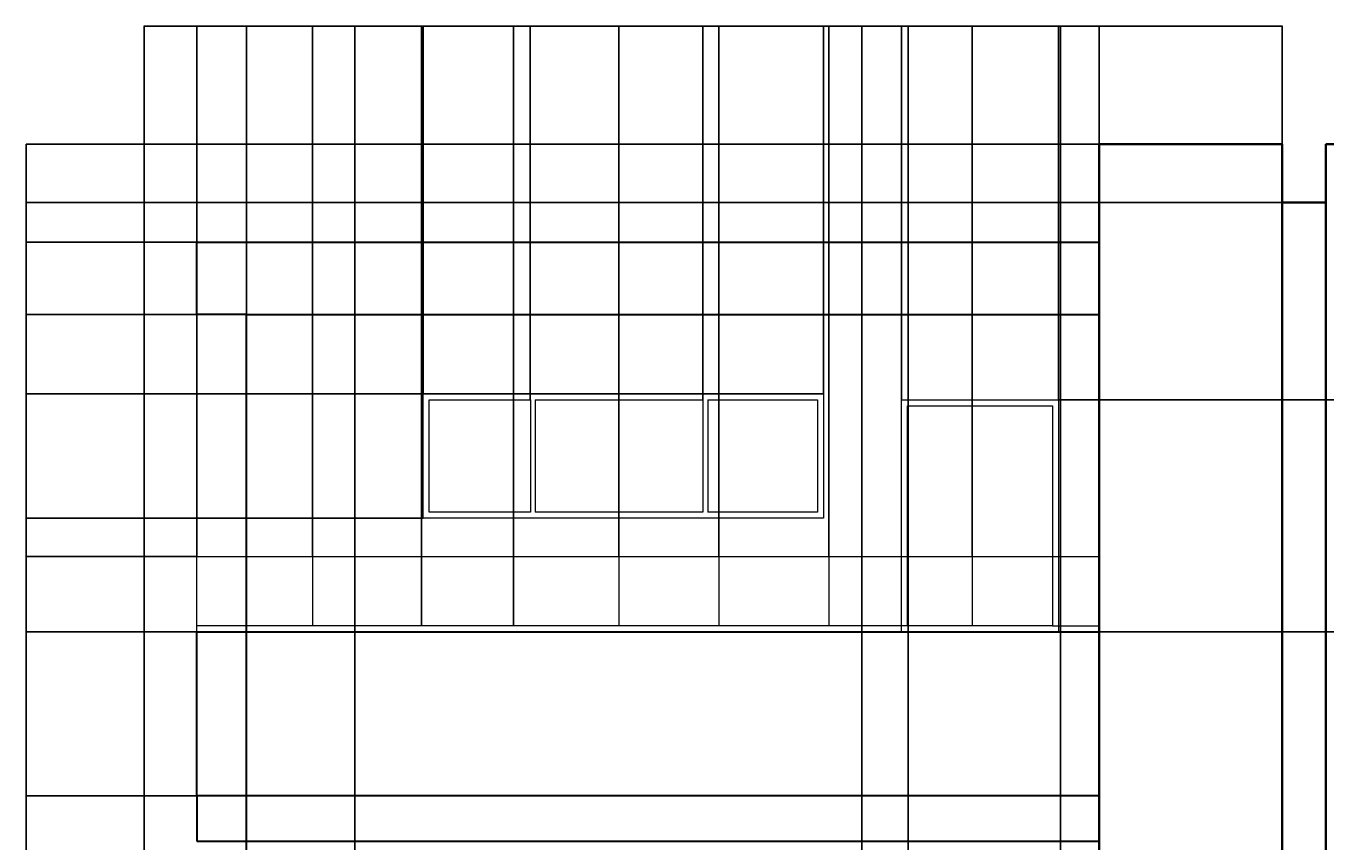
# Model space of a CAD drawing. Units: millimetres. Extents: x 1225 to 9865, y 11 to 4912.
# Tile 2 of 4: x 1225 to 5562, y 2192 to 4912. Entities that reach past the tile are written whole.
import ezdxf

# ---------------------------------------------------------------- set-up
doc = ezdxf.new("R2010")
doc.units = ezdxf.units.MM
for name, color, linetype, lineweight in [('A-ANNO-DIMS', 2, 'Continuous', 18), ('A-COLS', 7, 'Continuous', 35), ('A-DOOR', 3, 'Continuous', 20), ('A-FLOR', 7, 'Continuous', 30), ('A-FLOR-RAIL', 8, 'Continuous', 18), ('A-GLAZ', 4, 'Continuous', 18), ('A-ROOF', 7, 'Continuous', 30), ('A-WALL', 7, 'Continuous', 30)]:
    doc.layers.add(name, color=color, linetype=linetype, lineweight=lineweight)
doc.styles.get("Standard").update_dxf_attribs({"font": 'arial.ttf'})
doc.dimstyles.get("Standard").update_dxf_attribs({"dimtxt": 0.18, "dimasz": 0.18, "dimexe": 0.18, "dimexo": 0.0625, "dimgap": 0.09, "dimtad": 0, "dimtih": 1, "dimtoh": 1, "dimdec": 4, "dimzin": 0, "dimdsep": 46, "dimtxsty": 'Standard', "dimcen": 0.09, "dimadec": 0, "dimazin": 0, "dimtfac": 1, "dimtdec": 4, "dimtofl": 0, "dimtmove": 0, "dimatfit": 3, "dimfxl": 1, "dimtolj": 1, "dimtzin": 0, "dimarcsym": 0})

# ---------------------------------------------------------------- blocks, each defined once
blk = doc.blocks.new('*D2')
at = {"layer": 'A-ANNO-DIMS', "color": 0, "lineweight": -2, "transparency": 16777216}
for p, q in [((4805.3, 4517.6), (1225, 4517.6)), ((1225.2, 4517.4), (1225.2, 2461.4)), ((1225.2, 404.9), (1225.2, 2461)), ((1619.1, 404.8), (1225, 404.8))]:
    blk.add_line(p, q, dxfattribs=at)
at = {"layer": 'A-ANNO-DIMS', "color": 0, "transparency": 16777216}
for points in [[(1225.1, 4517.4), (1225.2, 4517.4), (1225.2, 4517.6)], [(1225.1, 404.9), (1225.2, 404.9), (1225.2, 404.8)]]:
    blk.add_solid(points, dxfattribs=at)
at = {"layer": 'Defpoints', "color": 0, "transparency": 16777216}
for p in [(1225.2, 4517.6), (4805.4, 4517.6), (1619.2, 404.8)]:
    blk.add_point(p, dxfattribs=at)
at = {"layer": 'A-ANNO-DIMS', "color": 0, "transparency": 16777216, "insert": (1225.2, 2461.2), "char_height": 0.18, "attachment_point": 5}
blk.add_mtext('\\A1;4113', dxfattribs=at)
blk = doc.blocks.new('*D3')
at = {"layer": 'A-ANNO-DIMS', "color": 0, "lineweight": -2, "transparency": 16777216}
for p, q in [((1619.2, 496.3), (1619.2, 4911.8)), ((1619.3, 4911.6), (1789.1, 4911.6)), ((1959.7, 4911.6), (1789.9, 4911.6)), ((1959.9, 496.3), (1959.9, 4911.8))]:
    blk.add_line(p, q, dxfattribs=at)
at = {"layer": 'A-ANNO-DIMS', "color": 0, "transparency": 16777216}
for points in [[(1619.3, 4911.6), (1619.3, 4911.6), (1619.2, 4911.6)], [(1959.7, 4911.6), (1959.7, 4911.6), (1959.9, 4911.6)]]:
    blk.add_solid(points, dxfattribs=at)
at = {"layer": 'Defpoints', "color": 0, "transparency": 16777216}
for p in [(1959.9, 4911.6), (1619.2, 496.3), (1959.9, 496.3)]:
    blk.add_point(p, dxfattribs=at)
at = {"layer": 'A-ANNO-DIMS', "color": 0, "transparency": 16777216, "insert": (1789.5, 4911.6), "char_height": 0.18, "attachment_point": 5}
blk.add_mtext('\\A1;340.7', dxfattribs=at)
blk = doc.blocks.new('*D4')
at = {"layer": 'A-ANNO-DIMS', "color": 0, "lineweight": -2, "transparency": 16777216}
for p, q in [((1959.9, 496.3), (1959.9, 4911.8)), ((1960.1, 4911.6), (2140.3, 4911.6)), ((2321.6, 4911.6), (2141.3, 4911.6)), ((2321.7, 496.3), (2321.7, 4911.8))]:
    blk.add_line(p, q, dxfattribs=at)
at = {"layer": 'A-ANNO-DIMS', "color": 0, "transparency": 16777216}
for points in [[(1960.1, 4911.6), (1960.1, 4911.6), (1959.9, 4911.6)], [(2321.6, 4911.6), (2321.6, 4911.6), (2321.7, 4911.6)]]:
    blk.add_solid(points, dxfattribs=at)
at = {"layer": 'Defpoints', "color": 0, "transparency": 16777216}
for p in [(2321.7, 4911.6), (1959.9, 496.3), (2321.7, 496.3)]:
    blk.add_point(p, dxfattribs=at)
at = {"layer": 'A-ANNO-DIMS', "color": 0, "transparency": 16777216, "insert": (2140.8, 4911.6), "char_height": 0.18, "attachment_point": 5}
blk.add_mtext('\\A1;361.84', dxfattribs=at)
blk = doc.blocks.new('*D5')
at = {"layer": 'A-ANNO-DIMS', "color": 0, "lineweight": -2, "transparency": 16777216}
for p, q in [((2321.7, 1491.6), (2321.7, 4911.8)), ((2321.9, 4911.6), (3167.3, 4911.6)), ((4013.5, 4911.6), (3168, 4911.6)), ((4013.6, 1491.6), (4013.6, 4911.8))]:
    blk.add_line(p, q, dxfattribs=at)
at = {"layer": 'A-ANNO-DIMS', "color": 0, "transparency": 16777216}
for points in [[(2321.9, 4911.6), (2321.9, 4911.6), (2321.7, 4911.6)], [(4013.5, 4911.6), (4013.5, 4911.6), (4013.6, 4911.6)]]:
    blk.add_solid(points, dxfattribs=at)
at = {"layer": 'Defpoints', "color": 0, "transparency": 16777216}
for p in [(4013.6, 4911.6), (2321.7, 1491.5), (4013.6, 1491.5)]:
    blk.add_point(p, dxfattribs=at)
at = {"layer": 'A-ANNO-DIMS', "color": 0, "transparency": 16777216, "insert": (3167.7, 4911.6), "char_height": 0.18, "attachment_point": 5}
blk.add_mtext('\\A1;1692', dxfattribs=at)
blk = doc.blocks.new('*D6')
at = {"layer": 'A-ANNO-DIMS', "color": 0, "lineweight": -2, "transparency": 16777216}
for p, q in [((4013.6, 1491.6), (4013.6, 4911.8)), ((4013.8, 4911.6), (4090.2, 4911.6)), ((4167.3, 4911.6), (4090.9, 4911.6)), ((4167.5, 1391.1), (4167.5, 4911.8))]:
    blk.add_line(p, q, dxfattribs=at)
at = {"layer": 'A-ANNO-DIMS', "color": 0, "transparency": 16777216}
for points in [[(4013.8, 4911.6), (4013.8, 4911.6), (4013.6, 4911.6)], [(4167.3, 4911.6), (4167.3, 4911.6), (4167.5, 4911.6)]]:
    blk.add_solid(points, dxfattribs=at)
at = {"layer": 'Defpoints', "color": 0, "transparency": 16777216}
for p in [(4167.5, 4911.6), (4013.6, 1491.5), (4167.5, 1391.1)]:
    blk.add_point(p, dxfattribs=at)
at = {"layer": 'A-ANNO-DIMS', "color": 0, "transparency": 16777216, "insert": (4090.5, 4911.6), "char_height": 0.18, "attachment_point": 5}
blk.add_mtext('\\A1;153.8', dxfattribs=at)
blk = doc.blocks.new('*D7')
at = {"layer": 'A-ANNO-DIMS', "color": 0, "lineweight": -2, "transparency": 16777216}
for p, q in [((4167.5, 1391.1), (4167.5, 4911.8)), ((4167.6, 4911.6), (4421.4, 4911.6)), ((4676, 4911.6), (4422.2, 4911.6)), ((4676.2, 1391.1), (4676.2, 4911.8))]:
    blk.add_line(p, q, dxfattribs=at)
at = {"layer": 'A-ANNO-DIMS', "color": 0, "transparency": 16777216}
for points in [[(4167.6, 4911.6), (4167.6, 4911.6), (4167.5, 4911.6)], [(4676, 4911.6), (4676, 4911.6), (4676.2, 4911.6)]]:
    blk.add_solid(points, dxfattribs=at)
at = {"layer": 'Defpoints', "color": 0, "transparency": 16777216}
for p in [(4676.2, 4911.6), (4167.5, 1391.1), (4676.2, 1391.1)]:
    blk.add_point(p, dxfattribs=at)
at = {"layer": 'A-ANNO-DIMS', "color": 0, "transparency": 16777216, "insert": (4421.8, 4911.6), "char_height": 0.18, "attachment_point": 5}
blk.add_mtext('\\A1;508.8', dxfattribs=at)
blk = doc.blocks.new('*D8')
at = {"layer": 'A-ANNO-DIMS', "color": 0, "lineweight": -2, "transparency": 16777216}
for p, q in [((4805.4, 4517.7), (4805.4, 4911.8)), ((4805.6, 4911.6), (5110.1, 4911.6)), ((5415.2, 4911.6), (5110.7, 4911.6)), ((5415.4, 4517.7), (5415.4, 4911.8))]:
    blk.add_line(p, q, dxfattribs=at)
at = {"layer": 'A-ANNO-DIMS', "color": 0, "transparency": 16777216}
for points in [[(4805.6, 4911.6), (4805.6, 4911.6), (4805.4, 4911.6)], [(5415.2, 4911.6), (5415.2, 4911.6), (5415.4, 4911.6)]]:
    blk.add_solid(points, dxfattribs=at)
at = {"layer": 'Defpoints', "color": 0, "transparency": 16777216}
for p in [(5415.4, 4911.6), (4805.4, 4517.6), (5415.4, 4517.6)]:
    blk.add_point(p, dxfattribs=at)
at = {"layer": 'A-ANNO-DIMS', "color": 0, "transparency": 16777216, "insert": (5110.4, 4911.6), "char_height": 0.18, "attachment_point": 5}
blk.add_mtext('\\A1;610', dxfattribs=at)
blk = doc.blocks.new('*D9')
at = {"layer": 'A-ANNO-DIMS', "color": 0, "lineweight": -2, "transparency": 16777216}
for p, q in [((5415.4, 4322.4), (5415.4, 10.6)), ((5561.8, 4322.4), (5561.8, 10.6)), ((5415.6, 10.8), (5488.1, 10.8)), ((5561.6, 10.8), (5489, 10.8))]:
    blk.add_line(p, q, dxfattribs=at)
at = {"layer": 'A-ANNO-DIMS', "color": 0, "transparency": 16777216}
for points in [[(5415.6, 10.8), (5415.6, 10.7), (5415.4, 10.8)], [(5561.6, 10.8), (5561.6, 10.7), (5561.8, 10.8)]]:
    blk.add_solid(points, dxfattribs=at)
at = {"layer": 'Defpoints', "color": 0, "transparency": 16777216}
for p in [(5415.4, 4322.4), (5561.8, 4322.4), (5561.8, 10.8)]:
    blk.add_point(p, dxfattribs=at)
at = {"layer": 'A-ANNO-DIMS', "color": 0, "transparency": 16777216, "insert": (5488.6, 10.8), "char_height": 0.18, "attachment_point": 5}
blk.add_mtext('\\A1;146.38', dxfattribs=at)
blk = doc.blocks.new('*D11')
at = {"layer": 'A-ANNO-DIMS', "color": 0, "lineweight": -2, "transparency": 16777216}
for p, q in [((5415.3, 4517.6), (1225, 4517.6)), ((1225.2, 4517.4), (1225.2, 4420.2)), ((1225.2, 4322.6), (1225.2, 4419.8)), ((5415.3, 4322.4), (1225, 4322.4))]:
    blk.add_line(p, q, dxfattribs=at)
at = {"layer": 'A-ANNO-DIMS', "color": 0, "transparency": 16777216}
for points in [[(1225.1, 4517.4), (1225.2, 4517.4), (1225.2, 4517.6)], [(1225.1, 4322.6), (1225.2, 4322.6), (1225.2, 4322.4)]]:
    blk.add_solid(points, dxfattribs=at)
at = {"layer": 'Defpoints', "color": 0, "transparency": 16777216}
for p in [(5415.4, 4517.6), (1225.2, 4322.4), (5415.4, 4322.4)]:
    blk.add_point(p, dxfattribs=at)
at = {"layer": 'A-ANNO-DIMS', "color": 0, "transparency": 16777216, "insert": (1225.2, 4420), "char_height": 0.18, "attachment_point": 5}
blk.add_mtext('\\A1;195.2', dxfattribs=at)
blk = doc.blocks.new('*D18')
at = {"layer": 'A-ANNO-DIMS', "color": 0, "lineweight": -2, "transparency": 16777216}
for p, q in [((1959.9, 3949.5), (1959.9, 4911.8)), ((1960.1, 4911.6), (3382.2, 4911.6)), ((4805.2, 4911.6), (3383.1, 4911.6)), ((4805.4, 4190.5), (4805.4, 4911.8))]:
    blk.add_line(p, q, dxfattribs=at)
at = {"layer": 'A-ANNO-DIMS', "color": 0, "transparency": 16777216}
for points in [[(1960.1, 4911.6), (1960.1, 4911.6), (1959.9, 4911.6)], [(4805.2, 4911.6), (4805.2, 4911.6), (4805.4, 4911.6)]]:
    blk.add_solid(points, dxfattribs=at)
at = {"layer": 'Defpoints', "color": 0, "transparency": 16777216}
for p in [(4805.4, 4911.6), (4805.4, 4190.5), (1959.9, 3949.4)]:
    blk.add_point(p, dxfattribs=at)
at = {"layer": 'A-ANNO-DIMS', "color": 0, "transparency": 16777216, "insert": (3382.6, 4911.6), "char_height": 0.18, "attachment_point": 5}
blk.add_mtext('\\A1;2845.5', dxfattribs=at)
blk = doc.blocks.new('*D21')
at = {"layer": 'A-ANNO-DIMS', "color": 0, "lineweight": -2, "transparency": 16777216}
for p, q in [((1794.2, 4190.5), (1794.2, 4911.8)), ((1794.4, 4911.6), (1876.6, 4911.6)), ((1959.7, 4911.6), (1877.5, 4911.6)), ((1959.9, 3949.5), (1959.9, 4911.8))]:
    blk.add_line(p, q, dxfattribs=at)
at = {"layer": 'A-ANNO-DIMS', "color": 0, "transparency": 16777216}
for points in [[(1794.4, 4911.6), (1794.4, 4911.6), (1794.2, 4911.6)], [(1959.7, 4911.6), (1959.7, 4911.6), (1959.9, 4911.6)]]:
    blk.add_solid(points, dxfattribs=at)
at = {"layer": 'Defpoints', "color": 0, "transparency": 16777216}
for p in [(1959.9, 4911.6), (1794.2, 4190.5), (1959.9, 3949.4)]:
    blk.add_point(p, dxfattribs=at)
at = {"layer": 'A-ANNO-DIMS', "color": 0, "transparency": 16777216, "insert": (1877.1, 4911.6), "char_height": 0.18, "attachment_point": 5}
blk.add_mtext('\\A1;165.68', dxfattribs=at)
blk = doc.blocks.new('*D22')
at = {"layer": 'A-ANNO-DIMS', "color": 0, "lineweight": -2, "transparency": 16777216}
for p, q in [((1959.9, 3949.5), (1959.9, 4911.8)), ((1960.1, 4911.6), (2254.3, 4911.6)), ((2549.2, 4911.6), (2255, 4911.6)), ((2549.4, 3684.7), (2549.4, 4911.8))]:
    blk.add_line(p, q, dxfattribs=at)
at = {"layer": 'A-ANNO-DIMS', "color": 0, "transparency": 16777216}
for points in [[(1960.1, 4911.6), (1960.1, 4911.6), (1959.9, 4911.6)], [(2549.2, 4911.6), (2549.2, 4911.6), (2549.4, 4911.6)]]:
    blk.add_solid(points, dxfattribs=at)
at = {"layer": 'Defpoints', "color": 0, "transparency": 16777216}
for p in [(2549.4, 4911.6), (1959.9, 3949.4), (2549.4, 3684.7)]:
    blk.add_point(p, dxfattribs=at)
at = {"layer": 'A-ANNO-DIMS', "color": 0, "transparency": 16777216, "insert": (2254.7, 4911.6), "char_height": 0.18, "attachment_point": 5}
blk.add_mtext('\\A1;589.5', dxfattribs=at)
blk = doc.blocks.new('*D23')
at = {"layer": 'A-ANNO-DIMS', "color": 0, "lineweight": -2, "transparency": 16777216}
for p, q in [((3884.9, 3684.7), (3884.9, 4911.8)), ((3885.1, 4911.6), (4014.9, 4911.6)), ((4145.5, 4911.6), (4015.7, 4911.6)), ((4145.7, 3664.7), (4145.7, 4911.8))]:
    blk.add_line(p, q, dxfattribs=at)
at = {"layer": 'A-ANNO-DIMS', "color": 0, "transparency": 16777216}
for points in [[(3885.1, 4911.6), (3885.1, 4911.6), (3884.9, 4911.6)], [(4145.5, 4911.6), (4145.5, 4911.6), (4145.7, 4911.6)]]:
    blk.add_solid(points, dxfattribs=at)
at = {"layer": 'Defpoints', "color": 0, "transparency": 16777216}
for p in [(4145.7, 4911.6), (3884.9, 3684.7), (4145.7, 3664.7)]:
    blk.add_point(p, dxfattribs=at)
at = {"layer": 'A-ANNO-DIMS', "color": 0, "transparency": 16777216, "insert": (4015.3, 4911.6), "char_height": 0.18, "attachment_point": 5}
blk.add_mtext('\\A1;260.8', dxfattribs=at)
blk = doc.blocks.new('*D24')
at = {"layer": 'A-ANNO-DIMS', "color": 0, "lineweight": -2, "transparency": 16777216}
for p, q in [((4145.7, 3664.7), (4145.7, 4911.8)), ((4145.9, 4911.6), (4406.9, 4911.6)), ((4668.8, 4911.6), (4407.7, 4911.6)), ((4668.9, 3664.7), (4668.9, 4911.8))]:
    blk.add_line(p, q, dxfattribs=at)
at = {"layer": 'A-ANNO-DIMS', "color": 0, "transparency": 16777216}
for points in [[(4145.9, 4911.6), (4145.9, 4911.6), (4145.7, 4911.6)], [(4668.8, 4911.6), (4668.8, 4911.6), (4668.9, 4911.6)]]:
    blk.add_solid(points, dxfattribs=at)
at = {"layer": 'Defpoints', "color": 0, "transparency": 16777216}
for p in [(4668.9, 4911.6), (4145.7, 3664.7), (4668.9, 3664.7)]:
    blk.add_point(p, dxfattribs=at)
at = {"layer": 'A-ANNO-DIMS', "color": 0, "transparency": 16777216, "insert": (4407.3, 4911.6), "char_height": 0.18, "attachment_point": 5}
blk.add_mtext('\\A1;523.2', dxfattribs=at)
blk = doc.blocks.new('*D31')
at = {"layer": 'A-ANNO-DIMS', "color": 0, "lineweight": -2, "transparency": 16777216}
for p, q in [((1794.1, 2889.7), (1225, 2889.7)), ((1225.2, 2889.5), (1225.2, 2616.5)), ((1225.2, 2343.2), (1225.2, 2616.2)), ((1794.1, 2343), (1225, 2343))]:
    blk.add_line(p, q, dxfattribs=at)
at = {"layer": 'A-ANNO-DIMS', "color": 0, "transparency": 16777216}
for points in [[(1225.1, 2889.5), (1225.2, 2889.5), (1225.2, 2889.7)], [(1225.1, 2343.2), (1225.2, 2343.2), (1225.2, 2343)]]:
    blk.add_solid(points, dxfattribs=at)
at = {"layer": 'Defpoints', "color": 0, "transparency": 16777216}
for p in [(1225.2, 2889.7), (1794.2, 2889.7), (1794.2, 2343)]:
    blk.add_point(p, dxfattribs=at)
at = {"layer": 'A-ANNO-DIMS', "color": 0, "transparency": 16777216, "insert": (1225.2, 2616.3), "char_height": 0.18, "attachment_point": 5}
blk.add_mtext('\\A1;546.7', dxfattribs=at)
blk = doc.blocks.new('*D32')
at = {"layer": 'A-ANNO-DIMS', "color": 0, "lineweight": -2, "transparency": 16777216}
for p, q in [((1794.1, 3141.6), (1225, 3141.6)), ((1225.2, 3141.4), (1225.2, 3015.8)), ((1225.2, 2889.9), (1225.2, 3015.5)), ((1794.1, 2889.7), (1225, 2889.7))]:
    blk.add_line(p, q, dxfattribs=at)
at = {"layer": 'A-ANNO-DIMS', "color": 0, "transparency": 16777216}
for points in [[(1225.1, 3141.4), (1225.2, 3141.4), (1225.2, 3141.6)], [(1225.1, 2889.9), (1225.2, 2889.9), (1225.2, 2889.7)]]:
    blk.add_solid(points, dxfattribs=at)
at = {"layer": 'Defpoints', "color": 0, "transparency": 16777216}
for p in [(1225.2, 3141.6), (1794.2, 3141.6), (1794.2, 2889.7)]:
    blk.add_point(p, dxfattribs=at)
at = {"layer": 'A-ANNO-DIMS', "color": 0, "transparency": 16777216, "insert": (1225.2, 3015.6), "char_height": 0.18, "attachment_point": 5}
blk.add_mtext('\\A1;251.9', dxfattribs=at)
blk = doc.blocks.new('*D33')
at = {"layer": 'A-ANNO-DIMS', "color": 0, "lineweight": -2, "transparency": 16777216}
for p, q in [((1794.1, 3949.4), (1225, 3949.4)), ((1225.2, 3949.2), (1225.2, 3545.7)), ((1225.2, 3141.8), (1225.2, 3545.3)), ((1794.1, 3141.6), (1225, 3141.6))]:
    blk.add_line(p, q, dxfattribs=at)
at = {"layer": 'A-ANNO-DIMS', "color": 0, "transparency": 16777216}
for points in [[(1225.1, 3949.2), (1225.2, 3949.2), (1225.2, 3949.4)], [(1225.1, 3141.8), (1225.2, 3141.8), (1225.2, 3141.6)]]:
    blk.add_solid(points, dxfattribs=at)
at = {"layer": 'Defpoints', "color": 0, "transparency": 16777216}
for p in [(1225.2, 3949.4), (1794.2, 3949.4), (1794.2, 3141.6)]:
    blk.add_point(p, dxfattribs=at)
at = {"layer": 'A-ANNO-DIMS', "color": 0, "transparency": 16777216, "insert": (1225.2, 3545.5), "char_height": 0.18, "attachment_point": 5}
blk.add_mtext('\\A1;807.8', dxfattribs=at)
blk = doc.blocks.new('*D34')
at = {"layer": 'A-ANNO-DIMS', "color": 0, "lineweight": -2, "transparency": 16777216}
for p, q in [((1794.1, 4190.5), (1225, 4190.5)), ((1225.2, 4190.3), (1225.2, 4070.1)), ((1225.2, 3949.6), (1225.2, 4069.7)), ((1794.1, 3949.4), (1225, 3949.4))]:
    blk.add_line(p, q, dxfattribs=at)
at = {"layer": 'A-ANNO-DIMS', "color": 0, "transparency": 16777216}
for points in [[(1225.1, 4190.3), (1225.2, 4190.3), (1225.2, 4190.5)], [(1225.1, 3949.6), (1225.2, 3949.6), (1225.2, 3949.4)]]:
    blk.add_solid(points, dxfattribs=at)
at = {"layer": 'Defpoints', "color": 0, "transparency": 16777216}
for p in [(1225.2, 4190.5), (1794.2, 4190.5), (1794.2, 3949.4)]:
    blk.add_point(p, dxfattribs=at)
at = {"layer": 'A-ANNO-DIMS', "color": 0, "transparency": 16777216, "insert": (1225.2, 4069.9), "char_height": 0.18, "attachment_point": 5}
blk.add_mtext('\\A1;241.05', dxfattribs=at)
blk = doc.blocks.new('*D35')
at = {"layer": 'A-ANNO-DIMS', "color": 0, "lineweight": -2, "transparency": 16777216}
for p, q in [((2549.4, 3684.7), (1225, 3684.7)), ((1225.2, 3684.5), (1225.2, 3477.3)), ((1225.2, 3269.7), (1225.2, 3476.9)), ((2549.4, 3269.5), (1225, 3269.5))]:
    blk.add_line(p, q, dxfattribs=at)
at = {"layer": 'A-ANNO-DIMS', "color": 0, "transparency": 16777216}
for points in [[(1225.1, 3684.5), (1225.2, 3684.5), (1225.2, 3684.7)], [(1225.1, 3269.7), (1225.2, 3269.7), (1225.2, 3269.5)]]:
    blk.add_solid(points, dxfattribs=at)
at = {"layer": 'Defpoints', "color": 0, "transparency": 16777216}
for p in [(2549.4, 3684.7), (1225.2, 3269.5), (2549.4, 3269.5)]:
    blk.add_point(p, dxfattribs=at)
at = {"layer": 'A-ANNO-DIMS', "color": 0, "transparency": 16777216, "insert": (1225.2, 3477.1), "char_height": 0.18, "attachment_point": 5}
blk.add_mtext('\\A1;415.1', dxfattribs=at)
blk = doc.blocks.new('*D36')
at = {"layer": 'A-ANNO-DIMS', "color": 0, "lineweight": -2, "transparency": 16777216}
for p, q in [((4805.3, 3949.4), (1225, 3949.4)), ((1225.2, 3949.2), (1225.2, 3817.2)), ((1225.2, 3684.8), (1225.2, 3816.8)), ((3884.8, 3684.7), (1225, 3684.7))]:
    blk.add_line(p, q, dxfattribs=at)
at = {"layer": 'A-ANNO-DIMS', "color": 0, "transparency": 16777216}
for points in [[(1225.1, 3949.2), (1225.2, 3949.2), (1225.2, 3949.4)], [(1225.1, 3684.8), (1225.2, 3684.8), (1225.2, 3684.7)]]:
    blk.add_solid(points, dxfattribs=at)
at = {"layer": 'Defpoints', "color": 0, "transparency": 16777216}
for p in [(1225.2, 3949.4), (4805.4, 3949.4), (3884.9, 3684.7)]:
    blk.add_point(p, dxfattribs=at)
at = {"layer": 'A-ANNO-DIMS', "color": 0, "transparency": 16777216, "insert": (1225.2, 3817), "char_height": 0.18, "attachment_point": 5}
blk.add_mtext('\\A1;264.73', dxfattribs=at)
blk = doc.blocks.new('*D37')
at = {"layer": 'A-ANNO-DIMS', "color": 0, "lineweight": -2, "transparency": 16777216}
for p, q in [((4669, 3664.7), (9864.4, 3664.7)), ((9864.3, 3664.5), (9864.3, 3277.4)), ((9864.3, 2889.9), (9864.3, 3277)), ((4669, 2889.7), (9864.4, 2889.7))]:
    blk.add_line(p, q, dxfattribs=at)
at = {"layer": 'A-ANNO-DIMS', "color": 0, "transparency": 16777216}
for points in [[(9864.2, 3664.5), (9864.3, 3664.5), (9864.3, 3664.7)], [(9864.2, 2889.9), (9864.3, 2889.9), (9864.3, 2889.7)]]:
    blk.add_solid(points, dxfattribs=at)
at = {"layer": 'Defpoints', "color": 0, "transparency": 16777216}
for p in [(4668.9, 3664.7), (9864.3, 3664.7), (4668.9, 2889.7)]:
    blk.add_point(p, dxfattribs=at)
at = {"layer": 'A-ANNO-DIMS', "color": 0, "transparency": 16777216, "insert": (9864.3, 3277.2), "char_height": 0.18, "attachment_point": 5}
blk.add_mtext('\\A1;775', dxfattribs=at)
blk = doc.blocks.new('*D45')
at = {"layer": 'A-ANNO-DIMS', "color": 0, "lineweight": -2, "transparency": 16777216}
for p, q in [((2549.4, 3684.7), (2549.4, 4911.8)), ((2549.6, 4911.6), (2728, 4911.6)), ((2907.2, 4911.6), (2728.8, 4911.6)), ((2907.3, 3664.7), (2907.3, 4911.8))]:
    blk.add_line(p, q, dxfattribs=at)
at = {"layer": 'A-ANNO-DIMS', "color": 0, "transparency": 16777216}
for points in [[(2549.6, 4911.6), (2549.6, 4911.6), (2549.4, 4911.6)], [(2907.2, 4911.6), (2907.2, 4911.6), (2907.3, 4911.6)]]:
    blk.add_solid(points, dxfattribs=at)
at = {"layer": 'Defpoints', "color": 0, "transparency": 16777216}
for p in [(2907.3, 4911.6), (2549.4, 3684.7), (2907.3, 3664.7)]:
    blk.add_point(p, dxfattribs=at)
at = {"layer": 'A-ANNO-DIMS', "color": 0, "transparency": 16777216, "insert": (2728.4, 4911.6), "char_height": 0.18, "attachment_point": 5}
blk.add_mtext('\\A1;357.9', dxfattribs=at)
blk = doc.blocks.new('*D46')
at = {"layer": 'A-ANNO-DIMS', "color": 0, "lineweight": -2, "transparency": 16777216}
for p, q in [((2907.3, 3664.7), (2907.3, 4911.8)), ((2907.5, 4911.6), (3194.6, 4911.6)), ((3482.2, 4911.6), (3195.2, 4911.6)), ((3482.4, 3664.7), (3482.4, 4911.8))]:
    blk.add_line(p, q, dxfattribs=at)
at = {"layer": 'A-ANNO-DIMS', "color": 0, "transparency": 16777216}
for points in [[(2907.5, 4911.6), (2907.5, 4911.6), (2907.3, 4911.6)], [(3482.2, 4911.6), (3482.2, 4911.6), (3482.4, 4911.6)]]:
    blk.add_solid(points, dxfattribs=at)
at = {"layer": 'Defpoints', "color": 0, "transparency": 16777216}
for p in [(3482.4, 4911.6), (2907.3, 3664.7), (3482.4, 3664.7)]:
    blk.add_point(p, dxfattribs=at)
at = {"layer": 'A-ANNO-DIMS', "color": 0, "transparency": 16777216, "insert": (3194.9, 4911.6), "char_height": 0.18, "attachment_point": 5}
blk.add_mtext('\\A1;575', dxfattribs=at)
blk = doc.blocks.new('*D47')
at = {"layer": 'A-ANNO-DIMS', "color": 0, "lineweight": -2, "transparency": 16777216}
for p, q in [((3482.4, 3664.7), (3482.4, 4911.8)), ((3482.6, 4911.6), (3683.2, 4911.6)), ((3884.7, 4911.6), (3684, 4911.6)), ((3884.9, 3684.7), (3884.9, 4911.8))]:
    blk.add_line(p, q, dxfattribs=at)
at = {"layer": 'A-ANNO-DIMS', "color": 0, "transparency": 16777216}
for points in [[(3482.6, 4911.6), (3482.6, 4911.6), (3482.4, 4911.6)], [(3884.7, 4911.6), (3884.7, 4911.6), (3884.9, 4911.6)]]:
    blk.add_solid(points, dxfattribs=at)
at = {"layer": 'Defpoints', "color": 0, "transparency": 16777216}
for p in [(3884.9, 4911.6), (3482.4, 3664.7), (3884.9, 3684.7)]:
    blk.add_point(p, dxfattribs=at)
at = {"layer": 'A-ANNO-DIMS', "color": 0, "transparency": 16777216, "insert": (3683.6, 4911.6), "char_height": 0.18, "attachment_point": 5}
blk.add_mtext('\\A1;402.5', dxfattribs=at)
blk = doc.blocks.new('*D55')
at = {"layer": 'A-ANNO-DIMS', "color": 0, "lineweight": -2, "transparency": 16777216}
for p, q in [((1794.2, 3141.7), (1794.2, 4911.8)), ((1794.4, 4911.6), (1987.3, 4911.6)), ((2180.9, 4911.6), (1988, 4911.6)), ((2181.1, 3141.7), (2181.1, 4911.8))]:
    blk.add_line(p, q, dxfattribs=at)
at = {"layer": 'A-ANNO-DIMS', "color": 0, "transparency": 16777216}
for points in [[(1794.4, 4911.6), (1794.4, 4911.6), (1794.2, 4911.6)], [(2180.9, 4911.6), (2180.9, 4911.6), (2181.1, 4911.6)]]:
    blk.add_solid(points, dxfattribs=at)
at = {"layer": 'Defpoints', "color": 0, "transparency": 16777216}
for p in [(2181.1, 4911.6), (1794.2, 3141.6), (2181.1, 3141.6)]:
    blk.add_point(p, dxfattribs=at)
at = {"layer": 'A-ANNO-DIMS', "color": 0, "transparency": 16777216, "insert": (1987.6, 4911.6), "char_height": 0.18, "attachment_point": 5}
blk.add_mtext('\\A1;386.9', dxfattribs=at)
blk = doc.blocks.new('*D56')
at = {"layer": 'A-ANNO-DIMS', "color": 0, "lineweight": -2, "transparency": 16777216}
for p, q in [((2181.1, 3141.7), (2181.1, 4911.8)), ((2181.3, 4911.6), (2362.4, 4911.6)), ((2544.5, 4911.6), (2363.3, 4911.6)), ((2544.6, 3141.7), (2544.6, 4911.8))]:
    blk.add_line(p, q, dxfattribs=at)
at = {"layer": 'A-ANNO-DIMS', "color": 0, "transparency": 16777216}
for points in [[(2181.3, 4911.6), (2181.3, 4911.6), (2181.1, 4911.6)], [(2544.5, 4911.6), (2544.5, 4911.6), (2544.6, 4911.6)]]:
    blk.add_solid(points, dxfattribs=at)
at = {"layer": 'Defpoints', "color": 0, "transparency": 16777216}
for p in [(2544.6, 4911.6), (2181.1, 3141.6), (2544.6, 3141.6)]:
    blk.add_point(p, dxfattribs=at)
at = {"layer": 'A-ANNO-DIMS', "color": 0, "transparency": 16777216, "insert": (2362.9, 4911.6), "char_height": 0.18, "attachment_point": 5}
blk.add_mtext('\\A1;363.56', dxfattribs=at)
blk = doc.blocks.new('*D57')
at = {"layer": 'A-ANNO-DIMS', "color": 0, "lineweight": -2, "transparency": 16777216}
for p, q in [((2544.6, 2909.7), (2544.6, 4911.8)), ((2544.8, 4911.6), (2697.3, 4911.6)), ((2850.6, 4911.6), (2698.2, 4911.6)), ((2850.8, 2909.7), (2850.8, 4911.8))]:
    blk.add_line(p, q, dxfattribs=at)
at = {"layer": 'A-ANNO-DIMS', "color": 0, "transparency": 16777216}
for points in [[(2544.8, 4911.6), (2544.8, 4911.6), (2544.6, 4911.6)], [(2850.6, 4911.6), (2850.6, 4911.6), (2850.8, 4911.6)]]:
    blk.add_solid(points, dxfattribs=at)
at = {"layer": 'Defpoints', "color": 0, "transparency": 16777216}
for p in [(2850.8, 4911.6), (2544.6, 2909.7), (2850.8, 2909.7)]:
    blk.add_point(p, dxfattribs=at)
at = {"layer": 'A-ANNO-DIMS', "color": 0, "transparency": 16777216, "insert": (2697.7, 4911.6), "char_height": 0.18, "attachment_point": 5}
blk.add_mtext('\\A1;306.16', dxfattribs=at)
blk = doc.blocks.new('*D58')
at = {"layer": 'A-ANNO-DIMS', "color": 0, "lineweight": -2, "transparency": 16777216}
for p, q in [((2850.8, 3141.7), (2850.8, 4911.8)), ((2851, 4911.6), (3026.5, 4911.6)), ((3202.7, 4911.6), (3027.2, 4911.6)), ((3202.9, 3141.7), (3202.9, 4911.8))]:
    blk.add_line(p, q, dxfattribs=at)
at = {"layer": 'A-ANNO-DIMS', "color": 0, "transparency": 16777216}
for points in [[(2851, 4911.6), (2851, 4911.6), (2850.8, 4911.6)], [(3202.7, 4911.6), (3202.7, 4911.6), (3202.9, 4911.6)]]:
    blk.add_solid(points, dxfattribs=at)
at = {"layer": 'Defpoints', "color": 0, "transparency": 16777216}
for p in [(3202.9, 4911.6), (2850.8, 3141.6), (3202.9, 3141.6)]:
    blk.add_point(p, dxfattribs=at)
at = {"layer": 'A-ANNO-DIMS', "color": 0, "transparency": 16777216, "insert": (3026.8, 4911.6), "char_height": 0.18, "attachment_point": 5}
blk.add_mtext('\\A1;352.1', dxfattribs=at)
blk = doc.blocks.new('*D59')
at = {"layer": 'A-ANNO-DIMS', "color": 0, "lineweight": -2, "transparency": 16777216}
for p, q in [((3202.9, 3141.7), (3202.9, 4911.8)), ((3203.1, 4911.6), (3368.9, 4911.6)), ((3535.6, 4911.6), (3369.8, 4911.6)), ((3535.8, 3141.7), (3535.8, 4911.8))]:
    blk.add_line(p, q, dxfattribs=at)
at = {"layer": 'A-ANNO-DIMS', "color": 0, "transparency": 16777216}
for points in [[(3203.1, 4911.6), (3203.1, 4911.6), (3202.9, 4911.6)], [(3535.6, 4911.6), (3535.6, 4911.6), (3535.8, 4911.6)]]:
    blk.add_solid(points, dxfattribs=at)
at = {"layer": 'Defpoints', "color": 0, "transparency": 16777216}
for p in [(3535.8, 4911.6), (3202.9, 3141.6), (3535.8, 3141.6)]:
    blk.add_point(p, dxfattribs=at)
at = {"layer": 'A-ANNO-DIMS', "color": 0, "transparency": 16777216, "insert": (3369.4, 4911.6), "char_height": 0.18, "attachment_point": 5}
blk.add_mtext('\\A1;332.95', dxfattribs=at)
blk = doc.blocks.new('*D60')
at = {"layer": 'A-ANNO-DIMS', "color": 0, "lineweight": -2, "transparency": 16777216}
for p, q in [((3535.8, 3141.7), (3535.8, 4911.8)), ((3536, 4911.6), (3719.1, 4911.6)), ((3903, 4911.6), (3719.9, 4911.6)), ((3903.2, 3141.7), (3903.2, 4911.8))]:
    blk.add_line(p, q, dxfattribs=at)
at = {"layer": 'A-ANNO-DIMS', "color": 0, "transparency": 16777216}
for points in [[(3536, 4911.6), (3536, 4911.6), (3535.8, 4911.6)], [(3903, 4911.6), (3903, 4911.6), (3903.2, 4911.6)]]:
    blk.add_solid(points, dxfattribs=at)
at = {"layer": 'Defpoints', "color": 0, "transparency": 16777216}
for p in [(3903.2, 4911.6), (3535.8, 3141.6), (3903.2, 3141.6)]:
    blk.add_point(p, dxfattribs=at)
at = {"layer": 'A-ANNO-DIMS', "color": 0, "transparency": 16777216, "insert": (3719.5, 4911.6), "char_height": 0.18, "attachment_point": 5}
blk.add_mtext('\\A1;367.4', dxfattribs=at)
blk = doc.blocks.new('*D61')
at = {"layer": 'A-ANNO-DIMS', "color": 0, "lineweight": -2, "transparency": 16777216}
for p, q in [((3903.2, 3141.7), (3903.2, 4911.8)), ((3903.4, 4911.6), (4142, 4911.6)), ((4381.4, 4911.6), (4142.8, 4911.6)), ((4381.6, 3141.7), (4381.6, 4911.8))]:
    blk.add_line(p, q, dxfattribs=at)
at = {"layer": 'A-ANNO-DIMS', "color": 0, "transparency": 16777216}
for points in [[(3903.4, 4911.6), (3903.4, 4911.6), (3903.2, 4911.6)], [(4381.4, 4911.6), (4381.4, 4911.6), (4381.6, 4911.6)]]:
    blk.add_solid(points, dxfattribs=at)
at = {"layer": 'Defpoints', "color": 0, "transparency": 16777216}
for p in [(4381.6, 4911.6), (3903.2, 3141.6), (4381.6, 3141.6)]:
    blk.add_point(p, dxfattribs=at)
at = {"layer": 'A-ANNO-DIMS', "color": 0, "transparency": 16777216, "insert": (4142.4, 4911.6), "char_height": 0.18, "attachment_point": 5}
blk.add_mtext('\\A1;478.4', dxfattribs=at)

msp = doc.modelspace()

# ---------------------------------------------------------------- linework, layer by layer
at = {"layer": 'A-COLS'}
for p, q in [((4805.396, 3949.397), (4805.396, 4517.596)), ((4805.396, 4517.596), (5415.376, 4517.596)), ((5415.376, 4517.596), (5415.376, 496.264)), ((5561.752, 496.264), (5561.752, 4517.596)), ((5561.752, 4517.596), (6059.917, 4517.596)), ((5415.376, 4322.413), (5561.752, 4322.413)), ((4805.396, 3949.397), (4805.396, 496.264))]:
    msp.add_line(p, q, dxfattribs=at)
at = {"layer": 'A-DOOR'}
for points in [[(4145.693, 3664.662), (4668.935, 3664.662), (4668.935, 2889.682), (4145.693, 2889.682)], [(4165.693, 3644.662), (4648.935, 3644.662), (4648.935, 2909.682), (4165.693, 2909.682)]]:
    msp.add_lwpolyline(points, close=True, dxfattribs=at)
at = {"layer": 'A-FLOR'}
for p, q in [((4805.396, 2342.982), (1794.21, 2342.982)), ((1794.21, 2342.982), (1794.21, 2192.169)), ((1794.21, 2192.169), (4805.396, 2192.169))]:
    msp.add_line(p, q, dxfattribs=at)
at = {"layer": 'A-FLOR-RAIL'}
for p, q in [((1794.21, 2889.682), (1794.21, 3141.602)), ((1794.21, 3141.602), (4805.396, 3141.602)), ((2181.085, 3141.602), (2181.085, 2909.682)), ((2544.646, 3141.602), (2544.646, 2909.682)), ((2850.803, 3141.602), (2850.803, 2909.682)), ((3202.883, 3141.602), (3202.883, 2909.682)), ((3535.829, 3141.602), (3535.829, 2909.682)), ((3903.217, 3141.602), (3903.217, 2909.682)), ((4381.587, 3141.602), (4381.587, 2909.682)), ((4165.693, 2909.682), (1794.21, 2909.682)), ((4648.935, 2909.682), (4805.396, 2909.682))]:
    msp.add_line(p, q, dxfattribs=at)
at = {"layer": 'A-GLAZ'}
for p, q in [((2907.348, 3664.662), (2907.348, 3289.542)), ((2923.732, 3664.662), (2923.732, 3289.542)), ((3482.405, 3664.662), (3482.405, 3289.542)), ((3499.577, 3664.662), (3499.577, 3289.542))]:
    msp.add_line(p, q, dxfattribs=at)
msp.add_lwpolyline([(2549.414, 3684.662), (3884.876, 3684.662), (3884.876, 3269.542), (2549.414, 3269.542)], close=True, dxfattribs=at)
for points in [[(2907.348, 3289.542), (2569.414, 3289.542), (2569.414, 3664.662), (2907.348, 3664.662)], [(2923.732, 3664.662), (3482.405, 3664.662)], [(3499.577, 3664.662), (3864.876, 3664.662), (3864.876, 3289.542), (3499.577, 3289.542)], [(3482.405, 3289.542), (2923.732, 3289.542)]]:
    msp.add_lwpolyline(points, dxfattribs=at)
at = {"layer": 'A-ROOF'}
for p, q in [((1794.21, 3949.397), (1794.21, 4190.451)), ((1794.21, 4190.451), (4805.396, 4190.451)), ((1959.893, 3949.397), (1794.21, 3949.397)), ((1959.893, 3949.397), (4805.396, 3949.397))]:
    msp.add_line(p, q, dxfattribs=at)
at = {"layer": 'A-WALL'}
for p, q in [((1959.893, 496.264), (1959.893, 3949.397)), ((1794.21, 2342.982), (1794.21, 2889.682)), ((1794.21, 2889.682), (4805.396, 2889.682)), ((4805.396, 2889.682), (4805.396, 2192.169))]:
    msp.add_line(p, q, dxfattribs=at)

# ---------------------------------------------------------------- dimensions: what is measured, and where the dimension line sits
at = {"layer": 'A-ANNO-DIMS'}
for base, p1, p2, override, picture, middle in [((1959.893, 4911.596), (1619.167, 496.264), (1959.893, 496.264), {"dimdec": 1, "dimlfac": 1, "dimrnd": 0, "dimzin": 0, "dimdsep": 46, "dimlunit": 2}, '*D3', (1789.53, 4911.596)), ((1959.893, 4911.596), (1794.21, 4190.451), (1959.893, 3949.397), {"dimdec": 2, "dimlfac": 1, "dimrnd": 0, "dimzin": 0, "dimdsep": 46, "dimlunit": 2}, '*D21', (1877.051, 4911.596)), ((2181.085, 4911.596), (1794.21, 3141.602), (2181.085, 3141.602), {"dimdec": 1, "dimlfac": 1, "dimrnd": 0, "dimzin": 0, "dimdsep": 46, "dimlunit": 2}, '*D55', (1987.647, 4911.596)), ((2321.73, 4911.596), (1959.893, 496.264), (2321.73, 496.264), {"dimdec": 2, "dimlfac": 1, "dimrnd": 0, "dimzin": 0, "dimdsep": 46, "dimlunit": 2}, '*D4', (2140.812, 4911.596)), ((4805.396, 4911.596), (1959.893, 3949.397), (4805.396, 4190.451), {"dimdec": 1, "dimlfac": 1, "dimrnd": 0, "dimzin": 0, "dimdsep": 46, "dimlunit": 2}, '*D18', (3382.645, 4911.596)), ((2549.414, 4911.596), (1959.893, 3949.397), (2549.414, 3684.662), {"dimdec": 1, "dimlfac": 1, "dimrnd": 0, "dimzin": 0, "dimdsep": 46, "dimlunit": 2}, '*D22', (2254.654, 4911.596)), ((2544.646, 4911.596), (2181.085, 3141.602), (2544.646, 3141.602), {"dimdec": 2, "dimlfac": 1, "dimrnd": 0, "dimzin": 0, "dimdsep": 46, "dimlunit": 2}, '*D56', (2362.866, 4911.596)), ((4013.642, 4911.596), (2321.73, 1491.543), (4013.642, 1491.543), {"dimdec": 0, "dimlfac": 1, "dimrnd": 0, "dimzin": 0, "dimdsep": 46, "dimlunit": 2}, '*D5', (3167.686, 4911.596)), ((2850.803, 4911.596), (2544.646, 2909.682), (2850.803, 2909.682), {"dimdec": 2, "dimlfac": 1, "dimrnd": 0, "dimzin": 0, "dimdsep": 46, "dimlunit": 2}, '*D57', (2697.725, 4911.596)), ((2907.348, 4911.596), (2549.414, 3684.662), (2907.348, 3664.662), {"dimdec": 1, "dimlfac": 1, "dimrnd": 0, "dimzin": 0, "dimdsep": 46, "dimlunit": 2}, '*D45', (2728.381, 4911.596)), ((3202.883, 4911.596), (2850.803, 3141.602), (3202.883, 3141.602), {"dimdec": 1, "dimlfac": 1, "dimrnd": 0, "dimzin": 0, "dimdsep": 46, "dimlunit": 2}, '*D58', (3026.843, 4911.596)), ((3482.405, 4911.596), (2907.348, 3664.662), (3482.405, 3664.662), {"dimdec": 0, "dimlfac": 1, "dimrnd": 0, "dimzin": 0, "dimdsep": 46, "dimlunit": 2}, '*D46', (3194.876, 4911.596)), ((3535.829, 4911.596), (3202.883, 3141.602), (3535.829, 3141.602), {"dimdec": 2, "dimlfac": 1, "dimrnd": 0, "dimzin": 0, "dimdsep": 46, "dimlunit": 2}, '*D59', (3369.356, 4911.596)), ((3884.876, 4911.596), (3482.405, 3664.662), (3884.876, 3684.662), {"dimdec": 1, "dimlfac": 1, "dimrnd": 0, "dimzin": 0, "dimdsep": 46, "dimlunit": 2}, '*D47', (3683.64, 4911.596)), ((3903.217, 4911.596), (3535.829, 3141.602), (3903.217, 3141.602), {"dimdec": 1, "dimlfac": 1, "dimrnd": 0, "dimzin": 0, "dimdsep": 46, "dimlunit": 2}, '*D60', (3719.523, 4911.596)), ((4145.693, 4911.596), (3884.876, 3684.662), (4145.693, 3664.662), {"dimdec": 1, "dimlfac": 1, "dimrnd": 0, "dimzin": 0, "dimdsep": 46, "dimlunit": 2}, '*D23', (4015.285, 4911.596)), ((4381.587, 4911.596), (3903.217, 3141.602), (4381.587, 3141.602), {"dimdec": 1, "dimlfac": 1, "dimrnd": 0, "dimzin": 0, "dimdsep": 46, "dimlunit": 2}, '*D61', (4142.402, 4911.596)), ((4167.452, 4911.596), (4013.642, 1491.543), (4167.452, 1391.062), {"dimdec": 1, "dimlfac": 1, "dimrnd": 0, "dimzin": 0, "dimdsep": 46, "dimlunit": 2}, '*D6', (4090.547, 4911.596)), ((4668.935, 4911.596), (4145.693, 3664.662), (4668.935, 3664.662), {"dimdec": 1, "dimlfac": 1, "dimrnd": 0, "dimzin": 0, "dimdsep": 46, "dimlunit": 2}, '*D24', (4407.314, 4911.596)), ((4676.209, 4911.596), (4167.452, 1391.062), (4676.209, 1391.062), {"dimdec": 1, "dimlfac": 1, "dimrnd": 0, "dimzin": 0, "dimdsep": 46, "dimlunit": 2}, '*D7', (4421.831, 4911.596)), ((5415.376, 4911.596), (4805.396, 4517.596), (5415.376, 4517.596), {"dimdec": 0, "dimlfac": 1, "dimrnd": 0, "dimzin": 0, "dimdsep": 46, "dimlunit": 2}, '*D8', (5110.386, 4911.596)), ((5561.752, 10.75), (5415.376, 4322.413), (5561.752, 4322.413), {"dimdec": 2, "dimlfac": 1, "dimrnd": 0, "dimzin": 0, "dimdsep": 46, "dimlunit": 2}, '*D9', (5488.564, 10.75))]:
    dim = msp.add_linear_dim(base=base, p1=p1, p2=p2, dimstyle='Standard', override=override, dxfattribs=at)
    dim.commit()
    dim.dimension.update_dxf_attribs({"geometry": picture, "text_midpoint": middle})
for base, p1, p2, override, picture, middle in [((1225.167, 4322.413), (5415.376, 4517.596), (5415.376, 4322.413), {"dimdec": 1, "dimlfac": 1, "dimrnd": 0, "dimzin": 0, "dimdsep": 46, "dimlunit": 2}, '*D11', (1225.167, 4420.005)), ((1225.167, 4517.596), (1619.167, 404.75), (4805.396, 4517.596), {"dimdec": 0, "dimlfac": 1, "dimrnd": 0, "dimzin": 0, "dimdsep": 46, "dimlunit": 2}, '*D2', (1225.167, 2461.173)), ((1225.167, 4190.451), (1794.21, 3949.397), (1794.21, 4190.451), {"dimdec": 2, "dimlfac": 1, "dimrnd": 0, "dimzin": 0, "dimdsep": 46, "dimlunit": 2}, '*D34', (1225.167, 4069.924)), ((1225.1671, 3949.3968), (3884.8762, 3684.6619), (4805.3962, 3949.3968), {"dimdec": 2, "dimlfac": 1, "dimrnd": 0, "dimzin": 0, "dimdsep": 46, "dimlunit": 2}, '*D36', (1225.1671, 3817.0294)), ((1225.167, 3949.397), (1794.21, 3141.602), (1794.21, 3949.397), {"dimdec": 1, "dimlfac": 1, "dimrnd": 0, "dimzin": 0, "dimdsep": 46, "dimlunit": 2}, '*D33', (1225.167, 3545.5)), ((1225.167, 3269.542), (2549.414, 3684.662), (2549.414, 3269.542), {"dimdec": 1, "dimlfac": 1, "dimrnd": 0, "dimzin": 0, "dimdsep": 46, "dimlunit": 2}, '*D35', (1225.167, 3477.102)), ((9864.268, 3664.662), (4668.935, 2889.682), (4668.935, 3664.662), {"dimdec": 0, "dimlfac": 1, "dimrnd": 0, "dimzin": 0, "dimdsep": 46, "dimlunit": 2}, '*D37', (9864.268, 3277.172)), ((1225.167, 3141.602), (1794.21, 2889.682), (1794.21, 3141.602), {"dimdec": 1, "dimlfac": 1, "dimrnd": 0, "dimzin": 0, "dimdsep": 46, "dimlunit": 2}, '*D32', (1225.167, 3015.642)), ((1225.167, 2889.682), (1794.21, 2342.982), (1794.21, 2889.682), {"dimdec": 1, "dimlfac": 1, "dimrnd": 0, "dimzin": 0, "dimdsep": 46, "dimlunit": 2}, '*D31', (1225.167, 2616.332))]:
    dim = msp.add_linear_dim(base=base, p1=p1, p2=p2, angle=90, dimstyle='Standard', override=override, dxfattribs=at)
    dim.commit()
    dim.dimension.update_dxf_attribs({"geometry": picture, "text_midpoint": middle})

doc.saveas('drawing.dxf')
